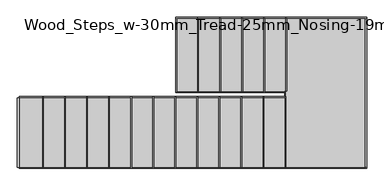
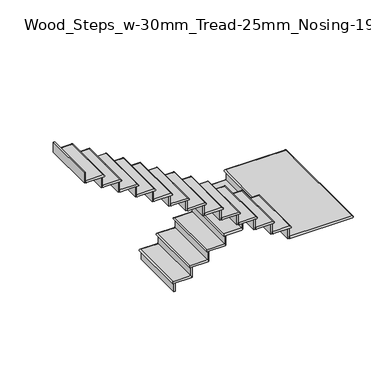
"""IFC4 building model written with IfcOpenShell, lengths in millimetres: stair flight geometry, Wood_Steps_w-30mm_Tread-25mm_Nosing-19mm_Riser."""

from ifc_helpers import new_model, si_unit, frame, origin, place, context, project, spatial, circle_curve, ellipse_curve, faceted_brep, source, transform, mapped, element, save
from ifc_brep_helpers import plane_surface, cylinder_surface, advanced_brep


def wood_steps_w_30mm_tread_25mm_nosing_19mm_riser_de9e5e1f(model_context):
    return source(origin(), model_context, "Body", "SolidModel", [
        advanced_brep(
        [(-8665.149573, -11058.3255223, 6797.52), (-8665.149573, -11058.3255223, 6827.52), (-8665.149573, -10219.6521308, 6827.52), (-8665.149573, -10219.6521308, 6797.52), (-8400.9545789, -11058.3255223, 6827.52), (-8400.9545789, -10219.6521308, 6827.52), (-8400.9545789, -10219.6521308, 6797.52), (-8400.9545789, -11058.3255223, 6797.52)],
        [
            (0, 1, ellipse_curve(frame((-8665.149573, -11058.3255223, 6812.52), z_axis=(-0.7071067811865475, 0.7071067811865475, 0.0), x_axis=(-0.7071067811865474, -0.7071067811865476, 0.0)), 21.2132034, 15.0)),
            (1, 2),
            (2, 3, ellipse_curve(frame((-8665.149573, -10219.6521308, 6812.52), z_axis=(-0.7071067811865475, -0.7071067811865475, 0.0), x_axis=(0.7071067811865474, -0.7071067811865476, 0.0)), 21.2132034, 15.0)),
            (3, 0),
            (4, 5),
            (5, 2),
            (1, 4),
            (6, 7),
            (7, 0),
            (3, 6),
            (4, 7, circle_curve(frame((-8400.9545789, -11058.3255223, 6812.52), z_axis=(1.0, 0.0, 0.0), x_axis=(0.0, 1.0, 0.0)), 15.0)),
            (6, 5, circle_curve(frame((-8400.9545789, -10219.6521308, 6812.52), z_axis=(1.0, 0.0, 0.0), x_axis=(0.0, -1.0, 0.0)), 15.0)),
        ],
        [
            cylinder_surface(frame((-8665.149573, -11058.3255223, 6812.52), z_axis=(0.0, -1.0, 0.0), x_axis=(1.0, 0.0, 0.0)), 15.0),
            plane_surface(frame((-6495.4132565, -10219.6521308, 6827.52), z_axis=(0.0, 0.0, 1.0), x_axis=(-1.0, 0.0, 0.0))),
            plane_surface(frame((-6495.4132565, -10219.6521308, 6797.52), z_axis=(0.0, 0.0, -1.0), x_axis=(1.0, 0.0, 0.0))),
            plane_surface(frame((-8400.9545789, -11058.3255223, 6827.52), z_axis=(1.0, 0.0, 0.0), x_axis=(0.0, 0.0, -1.0))),
            cylinder_surface(frame((-8400.9545789, -11058.3255223, 6812.52), z_axis=(1.0, 0.0, 0.0), x_axis=(0.0, 1.0, 0.0)), 15.0),
            cylinder_surface(frame((-8665.149573, -10219.6521308, 6812.52), z_axis=(-1.0, 0.0, 0.0), x_axis=(0.0, -1.0, 0.0)), 15.0),
        ],
        [
            (0, [[1, 2, 3, 4]]),
            (1, [[5, 6, -2, 7]]),
            (2, [[8, 9, -4, 10]]),
            (3, [[-5, 11, -8, 12]]),
            (4, [[-11, -7, -1, -9]]),
            (5, [[-3, -6, -12, -10]]),
        ],
    ),
        faceted_brep([(-8655.149573, -11058.3255223, 6797.52), (-8655.149573, -11058.3255223, 6664.96), (-8636.149573, -11058.3255223, 6664.96), (-8636.149573, -11058.3255223, 6797.52), (-8655.149573, -10219.6521308, 6797.52), (-8636.149573, -10219.6521308, 6797.52), (-8636.149573, -10219.6521308, 6664.96), (-8655.149573, -10219.6521308, 6664.96)], [[[0, 1, 2, 3]], [[4, 5, 6, 7]], [[1, 0, 4, 7]], [[2, 1, 7, 6]], [[3, 2, 6, 5]], [[0, 3, 5, 4]]]),
        faceted_brep([(-8400.9545789, -11058.3255223, 6960.08), (-8400.9545789, -11058.3255223, 6797.52), (-8381.9545789, -11058.3255223, 6797.52), (-8381.9545789, -11058.3255223, 6960.08), (-8400.9545789, -10219.6521308, 6960.08), (-8381.9545789, -10219.6521308, 6960.08), (-8381.9545789, -10219.6521308, 6797.52), (-8400.9545789, -10219.6521308, 6797.52)], [[[0, 1, 2, 3]], [[4, 5, 6, 7]], [[1, 0, 4, 7]], [[2, 1, 7, 6]], [[3, 2, 6, 5]], [[0, 3, 5, 4]]]),
        advanced_brep(
        [(-8146.7595849, -11058.3255223, 6990.08), (-8146.7595849, -10219.6521308, 6990.08), (-8410.9545789, -10219.6521308, 6990.08), (-8410.9545789, -11058.3255223, 6990.08), (-8146.7595849, -10219.6521308, 6960.08), (-8146.7595849, -11058.3255223, 6960.08), (-8410.9545789, -11058.3255223, 6960.08), (-8410.9545789, -10219.6521308, 6960.08)],
        [
            (0, 1),
            (1, 2),
            (2, 3),
            (3, 0),
            (4, 5),
            (5, 6),
            (6, 7),
            (7, 4),
            (0, 5, circle_curve(frame((-8146.7595849, -11058.3255223, 6975.08), z_axis=(1.0, 0.0, 0.0), x_axis=(0.0, 1.0, 0.0)), 15.0)),
            (4, 1, circle_curve(frame((-8146.7595849, -10219.6521308, 6975.08), z_axis=(1.0, 0.0, 0.0), x_axis=(0.0, -1.0, 0.0)), 15.0)),
            (6, 3, ellipse_curve(frame((-8410.9545789, -11058.3255223, 6975.08), z_axis=(-0.7071067811865475, 0.7071067811865475, 0.0), x_axis=(-0.7071067811865474, -0.7071067811865476, 0.0)), 21.2132034, 15.0)),
            (2, 7, ellipse_curve(frame((-8410.9545789, -10219.6521308, 6975.08), z_axis=(-0.7071067811865475, -0.7071067811865475, 0.0), x_axis=(0.7071067811865474, -0.7071067811865476, 0.0)), 21.2132034, 15.0)),
        ],
        [
            plane_surface(frame((-6495.4132565, -10219.6521308, 6990.08), z_axis=(0.0, 0.0, 1.0), x_axis=(-1.0, 0.0, 0.0))),
            plane_surface(frame((-6495.4132565, -10219.6521308, 6960.08), z_axis=(0.0, 0.0, -1.0), x_axis=(1.0, 0.0, 0.0))),
            plane_surface(frame((-8146.7595849, -11058.3255223, 6990.08), z_axis=(1.0, 0.0, 0.0), x_axis=(0.0, 0.0, -1.0))),
            cylinder_surface(frame((-8410.9545789, -11058.3255223, 6975.08), z_axis=(0.0, -1.0, 0.0), x_axis=(1.0, 0.0, 0.0)), 15.0),
            cylinder_surface(frame((-8146.7595849, -11058.3255223, 6975.08), z_axis=(1.0, 0.0, 0.0), x_axis=(0.0, 1.0, 0.0)), 15.0),
            cylinder_surface(frame((-8410.9545789, -10219.6521308, 6975.08), z_axis=(-1.0, 0.0, 0.0), x_axis=(0.0, -1.0, 0.0)), 15.0),
        ],
        [
            (0, [[1, 2, 3, 4]]),
            (1, [[5, 6, 7, 8]]),
            (2, [[-1, 9, -5, 10]]),
            (3, [[11, -3, 12, -7]]),
            (4, [[-9, -4, -11, -6]]),
            (5, [[-12, -2, -10, -8]]),
        ],
    ),
        faceted_brep([(-8146.7595849, -11058.3255223, 7122.64), (-8146.7595849, -11058.3255223, 6960.08), (-8127.7595849, -11058.3255223, 6960.08), (-8127.7595849, -11058.3255223, 7122.64), (-8146.7595849, -10219.6521308, 7122.64), (-8127.7595849, -10219.6521308, 7122.64), (-8127.7595849, -10219.6521308, 6960.08), (-8146.7595849, -10219.6521308, 6960.08)], [[[0, 1, 2, 3]], [[4, 5, 6, 7]], [[1, 0, 4, 7]], [[2, 1, 7, 6]], [[3, 2, 6, 5]], [[0, 3, 5, 4]]]),
        advanced_brep(
        [(-7893.1206135, -11058.3255223, 7152.64), (-7893.1206135, -10219.6521308, 7152.64), (-8156.7595849, -10219.6521308, 7152.64), (-8156.7595849, -11058.3255223, 7152.64), (-7893.1206135, -10219.6521308, 7122.64), (-7893.1206135, -11058.3255223, 7122.64), (-8156.7595849, -11058.3255223, 7122.64), (-8156.7595849, -10219.6521308, 7122.64)],
        [
            (0, 1),
            (1, 2),
            (2, 3),
            (3, 0),
            (4, 5),
            (5, 6),
            (6, 7),
            (7, 4),
            (0, 5, circle_curve(frame((-7893.1206135, -11058.3255223, 7137.64), z_axis=(1.0, 0.0, 0.0), x_axis=(0.0, 1.0, 0.0)), 15.0)),
            (4, 1, circle_curve(frame((-7893.1206135, -10219.6521308, 7137.64), z_axis=(1.0, 0.0, 0.0), x_axis=(0.0, -1.0, 0.0)), 15.0)),
            (6, 3, ellipse_curve(frame((-8156.7595849, -11058.3255223, 7137.64), z_axis=(-0.7071067811865475, 0.7071067811865475, 0.0), x_axis=(-0.7071067811865474, -0.7071067811865476, 0.0)), 21.2132034, 15.0)),
            (2, 7, ellipse_curve(frame((-8156.7595849, -10219.6521308, 7137.64), z_axis=(-0.7071067811865475, -0.7071067811865475, 0.0), x_axis=(0.7071067811865474, -0.7071067811865476, 0.0)), 21.2132034, 15.0)),
        ],
        [
            plane_surface(frame((-6495.4132565, -10219.6521308, 7152.64), z_axis=(0.0, 0.0, 1.0), x_axis=(-1.0, 0.0, 0.0))),
            plane_surface(frame((-6495.4132565, -10219.6521308, 7122.64), z_axis=(0.0, 0.0, -1.0), x_axis=(1.0, 0.0, 0.0))),
            plane_surface(frame((-7893.1206135, -11058.3255223, 7152.64), z_axis=(1.0, 0.0, 0.0), x_axis=(0.0, 0.0, -1.0))),
            cylinder_surface(frame((-8156.7595849, -11058.3255223, 7137.64), z_axis=(0.0, -1.0, 0.0), x_axis=(1.0, 0.0, 0.0)), 15.0),
            cylinder_surface(frame((-7893.1206135, -11058.3255223, 7137.64), z_axis=(1.0, 0.0, 0.0), x_axis=(0.0, 1.0, 0.0)), 15.0),
            cylinder_surface(frame((-8156.7595849, -10219.6521308, 7137.64), z_axis=(-1.0, 0.0, 0.0), x_axis=(0.0, -1.0, 0.0)), 15.0),
        ],
        [
            (0, [[1, 2, 3, 4]]),
            (1, [[5, 6, 7, 8]]),
            (2, [[-1, 9, -5, 10]]),
            (3, [[11, -3, 12, -7]]),
            (4, [[-9, -4, -11, -6]]),
            (5, [[-12, -2, -10, -8]]),
        ],
    ),
        faceted_brep([(-7893.1206135, -11058.3255223, 7285.2), (-7893.1206135, -11058.3255223, 7122.64), (-7874.1206135, -11058.3255223, 7122.64), (-7874.1206135, -11058.3255223, 7285.2), (-7893.1206135, -10219.6521308, 7285.2), (-7874.1206135, -10219.6521308, 7285.2), (-7874.1206135, -10219.6521308, 7122.64), (-7893.1206135, -10219.6521308, 7122.64)], [[[0, 1, 2, 3]], [[4, 5, 6, 7]], [[1, 0, 4, 7]], [[2, 1, 7, 6]], [[3, 2, 6, 5]], [[0, 3, 5, 4]]]),
        advanced_brep(
        [(-7638.9256194, -11058.3255223, 7315.2), (-7638.9256194, -10219.6521308, 7315.2), (-7903.1206135, -10219.6521308, 7315.2), (-7903.1206135, -11058.3255223, 7315.2), (-7638.9256194, -10219.6521308, 7285.2), (-7638.9256194, -11058.3255223, 7285.2), (-7903.1206135, -11058.3255223, 7285.2), (-7903.1206135, -10219.6521308, 7285.2)],
        [
            (0, 1),
            (1, 2),
            (2, 3),
            (3, 0),
            (4, 5),
            (5, 6),
            (6, 7),
            (7, 4),
            (0, 5, circle_curve(frame((-7638.9256194, -11058.3255223, 7300.2), z_axis=(1.0, 0.0, 0.0), x_axis=(0.0, 1.0, 0.0)), 15.0)),
            (4, 1, circle_curve(frame((-7638.9256194, -10219.6521308, 7300.2), z_axis=(1.0, 0.0, 0.0), x_axis=(0.0, -1.0, 0.0)), 15.0)),
            (6, 3, ellipse_curve(frame((-7903.1206135, -11058.3255223, 7300.2), z_axis=(-0.7071067811865475, 0.7071067811865475, 0.0), x_axis=(-0.7071067811865474, -0.7071067811865476, 0.0)), 21.2132034, 15.0)),
            (2, 7, ellipse_curve(frame((-7903.1206135, -10219.6521308, 7300.2), z_axis=(-0.7071067811865475, -0.7071067811865475, 0.0), x_axis=(0.7071067811865474, -0.7071067811865476, 0.0)), 21.2132034, 15.0)),
        ],
        [
            plane_surface(frame((-6495.4132565, -10219.6521308, 7315.2), z_axis=(0.0, 0.0, 1.0), x_axis=(-1.0, 0.0, 0.0))),
            plane_surface(frame((-6495.4132565, -10219.6521308, 7285.2), z_axis=(0.0, 0.0, -1.0), x_axis=(1.0, 0.0, 0.0))),
            plane_surface(frame((-7638.9256194, -11058.3255223, 7315.2), z_axis=(1.0, 0.0, 0.0), x_axis=(0.0, 0.0, -1.0))),
            cylinder_surface(frame((-7903.1206135, -11058.3255223, 7300.2), z_axis=(0.0, -1.0, 0.0), x_axis=(1.0, 0.0, 0.0)), 15.0),
            cylinder_surface(frame((-7638.9256194, -11058.3255223, 7300.2), z_axis=(1.0, 0.0, 0.0), x_axis=(0.0, 1.0, 0.0)), 15.0),
            cylinder_surface(frame((-7903.1206135, -10219.6521308, 7300.2), z_axis=(-1.0, 0.0, 0.0), x_axis=(0.0, -1.0, 0.0)), 15.0),
        ],
        [
            (0, [[1, 2, 3, 4]]),
            (1, [[5, 6, 7, 8]]),
            (2, [[-1, 9, -5, 10]]),
            (3, [[11, -3, 12, -7]]),
            (4, [[-9, -4, -11, -6]]),
            (5, [[-12, -2, -10, -8]]),
        ],
    ),
        faceted_brep([(-7384.7306254, -11058.3255223, 7610.32), (-7384.7306254, -11058.3255223, 7447.76), (-7365.7306254, -11058.3255223, 7447.76), (-7365.7306254, -11058.3255223, 7610.32), (-7384.7306254, -10219.6521308, 7610.32), (-7365.7306254, -10219.6521308, 7610.32), (-7365.7306254, -10219.6521308, 7447.76), (-7384.7306254, -10219.6521308, 7447.76)], [[[0, 1, 2, 3]], [[4, 5, 6, 7]], [[1, 0, 4, 7]], [[2, 1, 7, 6]], [[3, 2, 6, 5]], [[0, 3, 5, 4]]]),
        faceted_brep([(-7434.7306254, -11134.5255223, 7772.88), (-7434.7306254, -11134.5255223, 7610.32), (-7453.7306254, -11134.5255223, 7610.32), (-7453.7306254, -11134.5255223, 7772.88), (-7434.7306254, -11934.0860066, 7772.88), (-7453.7306254, -11934.0860066, 7772.88), (-7453.7306254, -11934.0860066, 7610.32), (-7434.7306254, -11934.0860066, 7610.32)], [[[0, 1, 2, 3]], [[4, 5, 6, 7]], [[1, 0, 4, 7]], [[2, 1, 7, 6]], [[3, 2, 6, 5]], [[0, 3, 5, 4]]]),
        advanced_brep(
        [(-7688.9256194, -11134.5255223, 7802.88), (-7688.9256194, -11934.0860066, 7802.88), (-7424.7306254, -11934.0860066, 7802.88), (-7424.7306254, -11134.5255223, 7802.88), (-7688.9256194, -11934.0860066, 7772.88), (-7688.9256194, -11134.5255223, 7772.88), (-7424.7306254, -11134.5255223, 7772.88), (-7424.7306254, -11934.0860066, 7772.88)],
        [
            (0, 1),
            (1, 2),
            (2, 3),
            (3, 0),
            (4, 5),
            (5, 6),
            (6, 7),
            (7, 4),
            (0, 5, circle_curve(frame((-7688.9256194, -11134.5255223, 7787.88), z_axis=(-1.0, 0.0, 0.0), x_axis=(0.0, -1.0, 0.0)), 15.0)),
            (4, 1, circle_curve(frame((-7688.9256194, -11934.0860066, 7787.88), z_axis=(-1.0, 0.0, 0.0), x_axis=(0.0, 1.0, 0.0)), 15.0)),
            (6, 3, ellipse_curve(frame((-7424.7306254, -11134.5255223, 7787.88), z_axis=(0.7071067811865475, -0.7071067811865475, 0.0), x_axis=(0.7071067811865474, 0.7071067811865476, 0.0)), 21.2132034, 15.0)),
            (2, 7, ellipse_curve(frame((-7424.7306254, -11934.0860066, 7787.88), z_axis=(0.7071067811865475, 0.7071067811865475, 0.0), x_axis=(-0.7071067811865474, 0.7071067811865476, 0.0)), 21.2132034, 15.0)),
        ],
        [
            plane_surface(frame((-10457.8773536, -11934.0860066, 7802.88), z_axis=(0.0, 0.0, 1.0), x_axis=(1.0, 0.0, 0.0))),
            plane_surface(frame((-10457.8773536, -11934.0860066, 7772.88), z_axis=(0.0, 0.0, -1.0), x_axis=(-1.0, 0.0, 0.0))),
            plane_surface(frame((-7688.9256194, -11134.5255223, 7802.88), z_axis=(-1.0, 0.0, 0.0), x_axis=(0.0, 0.0, -1.0))),
            cylinder_surface(frame((-7424.7306254, -11134.5255223, 7787.88), z_axis=(0.0, 1.0, 0.0), x_axis=(-1.0, 0.0, 0.0)), 15.0),
            cylinder_surface(frame((-7688.9256194, -11134.5255223, 7787.88), z_axis=(-1.0, 0.0, 0.0), x_axis=(0.0, -1.0, 0.0)), 15.0),
            cylinder_surface(frame((-7424.7306254, -11934.0860066, 7787.88), z_axis=(1.0, 0.0, 0.0), x_axis=(0.0, 1.0, 0.0)), 15.0),
        ],
        [
            (0, [[1, 2, 3, 4]]),
            (1, [[5, 6, 7, 8]]),
            (2, [[-1, 9, -5, 10]]),
            (3, [[11, -3, 12, -7]]),
            (4, [[-9, -4, -11, -6]]),
            (5, [[-12, -2, -10, -8]]),
        ],
    ),
        faceted_brep([(-8196.7595849, -11134.5255223, 8260.56), (-8196.7595849, -11134.5255223, 8098.0), (-8215.7595849, -11134.5255223, 8098.0), (-8215.7595849, -11134.5255223, 8260.56), (-8196.7595849, -11934.0860066, 8260.56), (-8215.7595849, -11934.0860066, 8260.56), (-8215.7595849, -11934.0860066, 8098.0), (-8196.7595849, -11934.0860066, 8098.0)], [[[0, 1, 2, 3]], [[4, 5, 6, 7]], [[1, 0, 4, 7]], [[2, 1, 7, 6]], [[3, 2, 6, 5]], [[0, 3, 5, 4]]]),
        advanced_brep(
        [(-8450.9545789, -11134.5255223, 8290.56), (-8450.9545789, -11934.0860066, 8290.56), (-8186.7595849, -11934.0860066, 8290.56), (-8186.7595849, -11134.5255223, 8290.56), (-8450.9545789, -11934.0860066, 8260.56), (-8450.9545789, -11134.5255223, 8260.56), (-8186.7595849, -11134.5255223, 8260.56), (-8186.7595849, -11934.0860066, 8260.56)],
        [
            (0, 1),
            (1, 2),
            (2, 3),
            (3, 0),
            (4, 5),
            (5, 6),
            (6, 7),
            (7, 4),
            (0, 5, circle_curve(frame((-8450.9545789, -11134.5255223, 8275.56), z_axis=(-1.0, 0.0, 0.0), x_axis=(0.0, -1.0, 0.0)), 15.0)),
            (4, 1, circle_curve(frame((-8450.9545789, -11934.0860066, 8275.56), z_axis=(-1.0, 0.0, 0.0), x_axis=(0.0, 1.0, 0.0)), 15.0)),
            (6, 3, ellipse_curve(frame((-8186.7595849, -11134.5255223, 8275.56), z_axis=(0.7071067811865475, -0.7071067811865475, 0.0), x_axis=(0.7071067811865474, 0.7071067811865476, 0.0)), 21.2132034, 15.0)),
            (2, 7, ellipse_curve(frame((-8186.7595849, -11934.0860066, 8275.56), z_axis=(0.7071067811865475, 0.7071067811865475, 0.0), x_axis=(-0.7071067811865474, 0.7071067811865476, 0.0)), 21.2132034, 15.0)),
        ],
        [
            plane_surface(frame((-10457.8773536, -11934.0860066, 8290.56), z_axis=(0.0, 0.0, 1.0), x_axis=(1.0, 0.0, 0.0))),
            plane_surface(frame((-10457.8773536, -11934.0860066, 8260.56), z_axis=(0.0, 0.0, -1.0), x_axis=(-1.0, 0.0, 0.0))),
            plane_surface(frame((-8450.9545789, -11134.5255223, 8290.56), z_axis=(-1.0, 0.0, 0.0), x_axis=(0.0, 0.0, -1.0))),
            cylinder_surface(frame((-8186.7595849, -11134.5255223, 8275.56), z_axis=(0.0, 1.0, 0.0), x_axis=(-1.0, 0.0, 0.0)), 15.0),
            cylinder_surface(frame((-8450.9545789, -11134.5255223, 8275.56), z_axis=(-1.0, 0.0, 0.0), x_axis=(0.0, -1.0, 0.0)), 15.0),
            cylinder_surface(frame((-8186.7595849, -11934.0860066, 8275.56), z_axis=(1.0, 0.0, 0.0), x_axis=(0.0, 1.0, 0.0)), 15.0),
        ],
        [
            (0, [[1, 2, 3, 4]]),
            (1, [[5, 6, 7, 8]]),
            (2, [[-1, 9, -5, 10]]),
            (3, [[11, -3, 12, -7]]),
            (4, [[-9, -4, -11, -6]]),
            (5, [[-12, -2, -10, -8]]),
        ],
    ),
        faceted_brep([(-8958.7885444, -11134.5255223, 8748.24), (-8958.7885444, -11134.5255223, 8585.68), (-8977.7885444, -11134.5255223, 8585.68), (-8977.7885444, -11134.5255223, 8748.24), (-8958.7885444, -11934.0860066, 8748.24), (-8977.7885444, -11934.0860066, 8748.24), (-8977.7885444, -11934.0860066, 8585.68), (-8958.7885444, -11934.0860066, 8585.68)], [[[0, 1, 2, 3]], [[4, 5, 6, 7]], [[1, 0, 4, 7]], [[2, 1, 7, 6]], [[3, 2, 6, 5]], [[0, 3, 5, 4]]]),
        advanced_brep(
        [(-9212.9835384, -11134.5255223, 8778.24), (-9212.9835384, -11934.0860066, 8778.24), (-8948.7885444, -11934.0860066, 8778.24), (-8948.7885444, -11134.5255223, 8778.24), (-9212.9835384, -11934.0860066, 8748.24), (-9212.9835384, -11134.5255223, 8748.24), (-8948.7885444, -11134.5255223, 8748.24), (-8948.7885444, -11934.0860066, 8748.24)],
        [
            (0, 1),
            (1, 2),
            (2, 3),
            (3, 0),
            (4, 5),
            (5, 6),
            (6, 7),
            (7, 4),
            (0, 5, circle_curve(frame((-9212.9835384, -11134.5255223, 8763.24), z_axis=(-1.0, 0.0, 0.0), x_axis=(0.0, -1.0, 0.0)), 15.0)),
            (4, 1, circle_curve(frame((-9212.9835384, -11934.0860066, 8763.24), z_axis=(-1.0, 0.0, 0.0), x_axis=(0.0, 1.0, 0.0)), 15.0)),
            (6, 3, ellipse_curve(frame((-8948.7885444, -11134.5255223, 8763.24), z_axis=(0.7071067811865475, -0.7071067811865475, 0.0), x_axis=(0.7071067811865474, 0.7071067811865476, 0.0)), 21.2132034, 15.0)),
            (2, 7, ellipse_curve(frame((-8948.7885444, -11934.0860066, 8763.24), z_axis=(0.7071067811865475, 0.7071067811865475, 0.0), x_axis=(-0.7071067811865474, 0.7071067811865476, 0.0)), 21.2132034, 15.0)),
        ],
        [
            plane_surface(frame((-10457.8773536, -11934.0860066, 8778.24), z_axis=(0.0, 0.0, 1.0), x_axis=(1.0, 0.0, 0.0))),
            plane_surface(frame((-10457.8773536, -11934.0860066, 8748.24), z_axis=(0.0, 0.0, -1.0), x_axis=(-1.0, 0.0, 0.0))),
            plane_surface(frame((-9212.9835384, -11134.5255223, 8778.24), z_axis=(-1.0, 0.0, 0.0), x_axis=(0.0, 0.0, -1.0))),
            cylinder_surface(frame((-8948.7885444, -11134.5255223, 8763.24), z_axis=(0.0, 1.0, 0.0), x_axis=(-1.0, 0.0, 0.0)), 15.0),
            cylinder_surface(frame((-9212.9835384, -11134.5255223, 8763.24), z_axis=(-1.0, 0.0, 0.0), x_axis=(0.0, -1.0, 0.0)), 15.0),
            cylinder_surface(frame((-8948.7885444, -11934.0860066, 8763.24), z_axis=(1.0, 0.0, 0.0), x_axis=(0.0, 1.0, 0.0)), 15.0),
        ],
        [
            (0, [[1, 2, 3, 4]]),
            (1, [[5, 6, 7, 8]]),
            (2, [[-1, 9, -5, 10]]),
            (3, [[11, -3, 12, -7]]),
            (4, [[-9, -4, -11, -6]]),
            (5, [[-12, -2, -10, -8]]),
        ],
    ),
        faceted_brep([(-9212.9835384, -11134.5255223, 8910.8), (-9212.9835384, -11134.5255223, 8748.24), (-9231.9835384, -11134.5255223, 8748.24), (-9231.9835384, -11134.5255223, 8910.8), (-9212.9835384, -11934.0860066, 8910.8), (-9231.9835384, -11934.0860066, 8910.8), (-9231.9835384, -11934.0860066, 8748.24), (-9212.9835384, -11934.0860066, 8748.24)], [[[0, 1, 2, 3]], [[4, 5, 6, 7]], [[1, 0, 4, 7]], [[2, 1, 7, 6]], [[3, 2, 6, 5]], [[0, 3, 5, 4]]]),
        advanced_brep(
        [(-9466.6534, -11134.5255223, 8940.8), (-9466.6534, -11934.0860066, 8940.8), (-9202.9835384, -11934.0860066, 8940.8), (-9202.9835384, -11134.5255223, 8940.8), (-9466.6534, -11934.0860066, 8910.8), (-9466.6534, -11134.5255223, 8910.8), (-9202.9835384, -11134.5255223, 8910.8), (-9202.9835384, -11934.0860066, 8910.8)],
        [
            (0, 1),
            (1, 2),
            (2, 3),
            (3, 0),
            (4, 5),
            (5, 6),
            (6, 7),
            (7, 4),
            (0, 5, circle_curve(frame((-9466.6534, -11134.5255223, 8925.8), z_axis=(-1.0, 0.0, 0.0), x_axis=(0.0, -1.0, 0.0)), 15.0)),
            (4, 1, circle_curve(frame((-9466.6534, -11934.0860066, 8925.8), z_axis=(-1.0, 0.0, 0.0), x_axis=(0.0, 1.0, 0.0)), 15.0)),
            (6, 3, ellipse_curve(frame((-9202.9835384, -11134.5255223, 8925.8), z_axis=(0.7071067811865475, -0.7071067811865475, 0.0), x_axis=(0.7071067811865474, 0.7071067811865476, 0.0)), 21.2132034, 15.0)),
            (2, 7, ellipse_curve(frame((-9202.9835384, -11934.0860066, 8925.8), z_axis=(0.7071067811865475, 0.7071067811865475, 0.0), x_axis=(-0.7071067811865474, 0.7071067811865476, 0.0)), 21.2132034, 15.0)),
        ],
        [
            plane_surface(frame((-10457.8773536, -11934.0860066, 8940.8), z_axis=(0.0, 0.0, 1.0), x_axis=(1.0, 0.0, 0.0))),
            plane_surface(frame((-10457.8773536, -11934.0860066, 8910.8), z_axis=(0.0, 0.0, -1.0), x_axis=(-1.0, 0.0, 0.0))),
            plane_surface(frame((-9466.6534, -11134.5255223, 8940.8), z_axis=(-1.0, 0.0, 0.0), x_axis=(0.0, 0.0, -1.0))),
            cylinder_surface(frame((-9202.9835384, -11134.5255223, 8925.8), z_axis=(0.0, 1.0, 0.0), x_axis=(-1.0, 0.0, 0.0)), 15.0),
            cylinder_surface(frame((-9466.6534, -11134.5255223, 8925.8), z_axis=(-1.0, 0.0, 0.0), x_axis=(0.0, -1.0, 0.0)), 15.0),
            cylinder_surface(frame((-9202.9835384, -11934.0860066, 8925.8), z_axis=(1.0, 0.0, 0.0), x_axis=(0.0, 1.0, 0.0)), 15.0),
        ],
        [
            (0, [[1, 2, 3, 4]]),
            (1, [[5, 6, 7, 8]]),
            (2, [[-1, 9, -5, 10]]),
            (3, [[11, -3, 12, -7]]),
            (4, [[-9, -4, -11, -6]]),
            (5, [[-12, -2, -10, -8]]),
        ],
    ),
        faceted_brep([(-9720.8175039, -11134.5255223, 9235.92), (-9720.8175039, -11134.5255223, 9073.36), (-9739.8175039, -11134.5255223, 9073.36), (-9739.8175039, -11134.5255223, 9235.92), (-9720.8175039, -11934.0860066, 9235.92), (-9739.8175039, -11934.0860066, 9235.92), (-9739.8175039, -11934.0860066, 9073.36), (-9720.8175039, -11934.0860066, 9073.36)], [[[0, 1, 2, 3]], [[4, 5, 6, 7]], [[1, 0, 4, 7]], [[2, 1, 7, 6]], [[3, 2, 6, 5]], [[0, 3, 5, 4]]]),
        advanced_brep(
        [(-9975.012498, -11134.5255223, 9265.92), (-9975.012498, -11934.0860066, 9265.92), (-9710.8175039, -11934.0860066, 9265.92), (-9710.8175039, -11134.5255223, 9265.92), (-9975.012498, -11934.0860066, 9235.92), (-9975.012498, -11134.5255223, 9235.92), (-9710.8175039, -11134.5255223, 9235.92), (-9710.8175039, -11934.0860066, 9235.92)],
        [
            (0, 1),
            (1, 2),
            (2, 3),
            (3, 0),
            (4, 5),
            (5, 6),
            (6, 7),
            (7, 4),
            (0, 5, circle_curve(frame((-9975.012498, -11134.5255223, 9250.92), z_axis=(-1.0, 0.0, 0.0), x_axis=(0.0, -1.0, 0.0)), 15.0)),
            (4, 1, circle_curve(frame((-9975.012498, -11934.0860066, 9250.92), z_axis=(-1.0, 0.0, 0.0), x_axis=(0.0, 1.0, 0.0)), 15.0)),
            (6, 3, ellipse_curve(frame((-9710.8175039, -11134.5255223, 9250.92), z_axis=(0.7071067811865475, -0.7071067811865475, 0.0), x_axis=(0.7071067811865474, 0.7071067811865476, 0.0)), 21.2132034, 15.0)),
            (2, 7, ellipse_curve(frame((-9710.8175039, -11934.0860066, 9250.92), z_axis=(0.7071067811865475, 0.7071067811865475, 0.0), x_axis=(-0.7071067811865474, 0.7071067811865476, 0.0)), 21.2132034, 15.0)),
        ],
        [
            plane_surface(frame((-10457.8773536, -11934.0860066, 9265.92), z_axis=(0.0, 0.0, 1.0), x_axis=(1.0, 0.0, 0.0))),
            plane_surface(frame((-10457.8773536, -11934.0860066, 9235.92), z_axis=(0.0, 0.0, -1.0), x_axis=(-1.0, 0.0, 0.0))),
            plane_surface(frame((-9975.012498, -11134.5255223, 9265.92), z_axis=(-1.0, 0.0, 0.0), x_axis=(0.0, 0.0, -1.0))),
            cylinder_surface(frame((-9710.8175039, -11134.5255223, 9250.92), z_axis=(0.0, 1.0, 0.0), x_axis=(-1.0, 0.0, 0.0)), 15.0),
            cylinder_surface(frame((-9975.012498, -11134.5255223, 9250.92), z_axis=(-1.0, 0.0, 0.0), x_axis=(0.0, -1.0, 0.0)), 15.0),
            cylinder_surface(frame((-9710.8175039, -11934.0860066, 9250.92), z_axis=(1.0, 0.0, 0.0), x_axis=(0.0, 1.0, 0.0)), 15.0),
        ],
        [
            (0, [[1, 2, 3, 4]]),
            (1, [[5, 6, 7, 8]]),
            (2, [[-1, 9, -5, 10]]),
            (3, [[11, -3, 12, -7]]),
            (4, [[-9, -4, -11, -6]]),
            (5, [[-12, -2, -10, -8]]),
        ],
    ),
        faceted_brep([(-9975.012498, -11134.5255223, 9398.48), (-9975.012498, -11134.5255223, 9235.92), (-9994.012498, -11134.5255223, 9235.92), (-9994.012498, -11134.5255223, 9398.48), (-9975.012498, -11934.0860066, 9398.48), (-9994.012498, -11934.0860066, 9398.48), (-9994.012498, -11934.0860066, 9235.92), (-9975.012498, -11934.0860066, 9235.92)], [[[0, 1, 2, 3]], [[4, 5, 6, 7]], [[1, 0, 4, 7]], [[2, 1, 7, 6]], [[3, 2, 6, 5]], [[0, 3, 5, 4]]]),
        advanced_brep(
        [(-10228.6823595, -11134.5255223, 9428.48), (-10228.6823595, -11934.0860066, 9428.48), (-9965.012498, -11934.0860066, 9428.48), (-9965.012498, -11134.5255223, 9428.48), (-10228.6823595, -11934.0860066, 9398.48), (-10228.6823595, -11134.5255223, 9398.48), (-9965.012498, -11134.5255223, 9398.48), (-9965.012498, -11934.0860066, 9398.48)],
        [
            (0, 1),
            (1, 2),
            (2, 3),
            (3, 0),
            (4, 5),
            (5, 6),
            (6, 7),
            (7, 4),
            (0, 5, circle_curve(frame((-10228.6823595, -11134.5255223, 9413.48), z_axis=(-1.0, 0.0, 0.0), x_axis=(0.0, -1.0, 0.0)), 15.0)),
            (4, 1, circle_curve(frame((-10228.6823595, -11934.0860066, 9413.48), z_axis=(-1.0, 0.0, 0.0), x_axis=(0.0, 1.0, 0.0)), 15.0)),
            (6, 3, ellipse_curve(frame((-9965.012498, -11134.5255223, 9413.48), z_axis=(0.7071067811865475, -0.7071067811865475, 0.0), x_axis=(0.7071067811865474, 0.7071067811865476, 0.0)), 21.2132034, 15.0)),
            (2, 7, ellipse_curve(frame((-9965.012498, -11934.0860066, 9413.48), z_axis=(0.7071067811865475, 0.7071067811865475, 0.0), x_axis=(-0.7071067811865474, 0.7071067811865476, 0.0)), 21.2132034, 15.0)),
        ],
        [
            plane_surface(frame((-10457.8773536, -11934.0860066, 9428.48), z_axis=(0.0, 0.0, 1.0), x_axis=(1.0, 0.0, 0.0))),
            plane_surface(frame((-10457.8773536, -11934.0860066, 9398.48), z_axis=(0.0, 0.0, -1.0), x_axis=(-1.0, 0.0, 0.0))),
            plane_surface(frame((-10228.6823595, -11134.5255223, 9428.48), z_axis=(-1.0, 0.0, 0.0), x_axis=(0.0, 0.0, -1.0))),
            cylinder_surface(frame((-9965.012498, -11134.5255223, 9413.48), z_axis=(0.0, 1.0, 0.0), x_axis=(-1.0, 0.0, 0.0)), 15.0),
            cylinder_surface(frame((-10228.6823595, -11134.5255223, 9413.48), z_axis=(-1.0, 0.0, 0.0), x_axis=(0.0, -1.0, 0.0)), 15.0),
            cylinder_surface(frame((-9965.012498, -11934.0860066, 9413.48), z_axis=(1.0, 0.0, 0.0), x_axis=(0.0, 1.0, 0.0)), 15.0),
        ],
        [
            (0, [[1, 2, 3, 4]]),
            (1, [[5, 6, 7, 8]]),
            (2, [[-1, 9, -5, 10]]),
            (3, [[11, -3, 12, -7]]),
            (4, [[-9, -4, -11, -6]]),
            (5, [[-12, -2, -10, -8]]),
        ],
    ),
        faceted_brep([(-10482.8773536, -11134.5255223, 9723.6), (-10482.8773536, -11134.5255223, 9561.04), (-10501.8773536, -11134.5255223, 9561.04), (-10501.8773536, -11134.5255223, 9723.6), (-10482.8773536, -11934.0860066, 9723.6), (-10501.8773536, -11934.0860066, 9723.6), (-10501.8773536, -11934.0860066, 9561.04), (-10482.8773536, -11934.0860066, 9561.04)], [[[0, 1, 2, 3]], [[4, 5, 6, 7]], [[1, 0, 4, 7]], [[2, 1, 7, 6]], [[3, 2, 6, 5]], [[0, 3, 5, 4]]]),
        faceted_brep([(-7638.9256194, -11058.3255223, 7447.76), (-7638.9256194, -11058.3255223, 7285.2), (-7619.9256194, -11058.3255223, 7285.2), (-7619.9256194, -11058.3255223, 7447.76), (-7638.9256194, -10219.6521308, 7447.76), (-7619.9256194, -10219.6521308, 7447.76), (-7619.9256194, -10219.6521308, 7285.2), (-7638.9256194, -10219.6521308, 7285.2)], [[[0, 1, 2, 3]], [[4, 5, 6, 7]], [[1, 0, 4, 7]], [[2, 1, 7, 6]], [[3, 2, 6, 5]], [[0, 3, 5, 4]]]),
        advanced_brep(
        [(-7384.7306254, -11058.3255223, 7477.76), (-7384.7306254, -10219.6521308, 7477.76), (-7648.9256194, -10219.6521308, 7477.76), (-7648.9256194, -11058.3255223, 7477.76), (-7384.7306254, -10219.6521308, 7447.76), (-7384.7306254, -11058.3255223, 7447.76), (-7648.9256194, -11058.3255223, 7447.76), (-7648.9256194, -10219.6521308, 7447.76)],
        [
            (0, 1),
            (1, 2),
            (2, 3),
            (3, 0),
            (4, 5),
            (5, 6),
            (6, 7),
            (7, 4),
            (0, 5, circle_curve(frame((-7384.7306254, -11058.3255223, 7462.76), z_axis=(1.0, 0.0, 0.0), x_axis=(0.0, 1.0, 0.0)), 15.0)),
            (4, 1, circle_curve(frame((-7384.7306254, -10219.6521308, 7462.76), z_axis=(1.0, 0.0, 0.0), x_axis=(0.0, -1.0, 0.0)), 15.0)),
            (6, 3, ellipse_curve(frame((-7648.9256194, -11058.3255223, 7462.76), z_axis=(-0.7071067811865475, 0.7071067811865475, 0.0), x_axis=(-0.7071067811865474, -0.7071067811865476, 0.0)), 21.2132034, 15.0)),
            (2, 7, ellipse_curve(frame((-7648.9256194, -10219.6521308, 7462.76), z_axis=(-0.7071067811865475, -0.7071067811865475, 0.0), x_axis=(0.7071067811865474, -0.7071067811865476, 0.0)), 21.2132034, 15.0)),
        ],
        [
            plane_surface(frame((-6241.2182625, -10219.6521308, 7477.76), z_axis=(0.0, 0.0, 1.0), x_axis=(-1.0, 0.0, 0.0))),
            plane_surface(frame((-6241.2182625, -10219.6521308, 7447.76), z_axis=(0.0, 0.0, -1.0), x_axis=(1.0, 0.0, 0.0))),
            plane_surface(frame((-7384.7306254, -11058.3255223, 7477.76), z_axis=(1.0, 0.0, 0.0), x_axis=(0.0, 0.0, -1.0))),
            cylinder_surface(frame((-7648.9256194, -11058.3255223, 7462.76), z_axis=(0.0, -1.0, 0.0), x_axis=(1.0, 0.0, 0.0)), 15.0),
            cylinder_surface(frame((-7384.7306254, -11058.3255223, 7462.76), z_axis=(1.0, 0.0, 0.0), x_axis=(0.0, 1.0, 0.0)), 15.0),
            cylinder_surface(frame((-7648.9256194, -10219.6521308, 7462.76), z_axis=(-1.0, 0.0, 0.0), x_axis=(0.0, -1.0, 0.0)), 15.0),
        ],
        [
            (0, [[1, 2, 3, 4]]),
            (1, [[5, 6, 7, 8]]),
            (2, [[-1, 9, -5, 10]]),
            (3, [[11, -3, 12, -7]]),
            (4, [[-9, -4, -11, -6]]),
            (5, [[-12, -2, -10, -8]]),
        ],
    ),
        faceted_brep([(-7688.9256194, -11134.5255223, 7935.44), (-7688.9256194, -11134.5255223, 7772.88), (-7707.9256194, -11134.5255223, 7772.88), (-7707.9256194, -11134.5255223, 7935.44), (-7688.9256194, -11934.0860066, 7935.44), (-7707.9256194, -11934.0860066, 7935.44), (-7707.9256194, -11934.0860066, 7772.88), (-7688.9256194, -11934.0860066, 7772.88)], [[[0, 1, 2, 3]], [[4, 5, 6, 7]], [[1, 0, 4, 7]], [[2, 1, 7, 6]], [[3, 2, 6, 5]], [[0, 3, 5, 4]]]),
        advanced_brep(
        [(-7943.1206135, -11134.5255223, 7965.44), (-7943.1206135, -11934.0860066, 7965.44), (-7678.9256194, -11934.0860066, 7965.44), (-7678.9256194, -11134.5255223, 7965.44), (-7943.1206135, -11934.0860066, 7935.44), (-7943.1206135, -11134.5255223, 7935.44), (-7678.9256194, -11134.5255223, 7935.44), (-7678.9256194, -11934.0860066, 7935.44)],
        [
            (0, 1),
            (1, 2),
            (2, 3),
            (3, 0),
            (4, 5),
            (5, 6),
            (6, 7),
            (7, 4),
            (0, 5, circle_curve(frame((-7943.1206135, -11134.5255223, 7950.44), z_axis=(-1.0, 0.0, 0.0), x_axis=(0.0, -1.0, 0.0)), 15.0)),
            (4, 1, circle_curve(frame((-7943.1206135, -11934.0860066, 7950.44), z_axis=(-1.0, 0.0, 0.0), x_axis=(0.0, 1.0, 0.0)), 15.0)),
            (6, 3, ellipse_curve(frame((-7678.9256194, -11134.5255223, 7950.44), z_axis=(0.7071067811865475, -0.7071067811865475, 0.0), x_axis=(0.7071067811865474, 0.7071067811865476, 0.0)), 21.2132034, 15.0)),
            (2, 7, ellipse_curve(frame((-7678.9256194, -11934.0860066, 7950.44), z_axis=(0.7071067811865475, 0.7071067811865475, 0.0), x_axis=(-0.7071067811865474, 0.7071067811865476, 0.0)), 21.2132034, 15.0)),
        ],
        [
            plane_surface(frame((-10712.0723476, -11934.0860066, 7965.44), z_axis=(0.0, 0.0, 1.0), x_axis=(1.0, 0.0, 0.0))),
            plane_surface(frame((-10712.0723476, -11934.0860066, 7935.44), z_axis=(0.0, 0.0, -1.0), x_axis=(-1.0, 0.0, 0.0))),
            plane_surface(frame((-7943.1206135, -11134.5255223, 7965.44), z_axis=(-1.0, 0.0, 0.0), x_axis=(0.0, 0.0, -1.0))),
            cylinder_surface(frame((-7678.9256194, -11134.5255223, 7950.44), z_axis=(0.0, 1.0, 0.0), x_axis=(-1.0, 0.0, 0.0)), 15.0),
            cylinder_surface(frame((-7943.1206135, -11134.5255223, 7950.44), z_axis=(-1.0, 0.0, 0.0), x_axis=(0.0, -1.0, 0.0)), 15.0),
            cylinder_surface(frame((-7678.9256194, -11934.0860066, 7950.44), z_axis=(1.0, 0.0, 0.0), x_axis=(0.0, 1.0, 0.0)), 15.0),
        ],
        [
            (0, [[1, 2, 3, 4]]),
            (1, [[5, 6, 7, 8]]),
            (2, [[-1, 9, -5, 10]]),
            (3, [[11, -3, 12, -7]]),
            (4, [[-9, -4, -11, -6]]),
            (5, [[-12, -2, -10, -8]]),
        ],
    ),
        faceted_brep([(-7943.1206135, -11134.5255223, 8098.0), (-7943.1206135, -11134.5255223, 7935.44), (-7962.1206135, -11134.5255223, 7935.44), (-7962.1206135, -11134.5255223, 8098.0), (-7943.1206135, -11934.0860066, 8098.0), (-7962.1206135, -11934.0860066, 8098.0), (-7962.1206135, -11934.0860066, 7935.44), (-7943.1206135, -11934.0860066, 7935.44)], [[[0, 1, 2, 3]], [[4, 5, 6, 7]], [[1, 0, 4, 7]], [[2, 1, 7, 6]], [[3, 2, 6, 5]], [[0, 3, 5, 4]]]),
        advanced_brep(
        [(-8196.7595849, -11134.5255223, 8128.0), (-8196.7595849, -11934.0860066, 8128.0), (-7933.1206135, -11934.0860066, 8128.0), (-7933.1206135, -11134.5255223, 8128.0), (-8196.7595849, -11934.0860066, 8098.0), (-8196.7595849, -11134.5255223, 8098.0), (-7933.1206135, -11134.5255223, 8098.0), (-7933.1206135, -11934.0860066, 8098.0)],
        [
            (0, 1),
            (1, 2),
            (2, 3),
            (3, 0),
            (4, 5),
            (5, 6),
            (6, 7),
            (7, 4),
            (0, 5, circle_curve(frame((-8196.7595849, -11134.5255223, 8113.0), z_axis=(-1.0, 0.0, 0.0), x_axis=(0.0, -1.0, 0.0)), 15.0)),
            (4, 1, circle_curve(frame((-8196.7595849, -11934.0860066, 8113.0), z_axis=(-1.0, 0.0, 0.0), x_axis=(0.0, 1.0, 0.0)), 15.0)),
            (6, 3, ellipse_curve(frame((-7933.1206135, -11134.5255223, 8113.0), z_axis=(0.7071067811865475, -0.7071067811865475, 0.0), x_axis=(0.7071067811865474, 0.7071067811865476, 0.0)), 21.2132034, 15.0)),
            (2, 7, ellipse_curve(frame((-7933.1206135, -11934.0860066, 8113.0), z_axis=(0.7071067811865475, 0.7071067811865475, 0.0), x_axis=(-0.7071067811865474, 0.7071067811865476, 0.0)), 21.2132034, 15.0)),
        ],
        [
            plane_surface(frame((-10457.8773536, -11934.0860066, 8128.0), z_axis=(0.0, 0.0, 1.0), x_axis=(1.0, 0.0, 0.0))),
            plane_surface(frame((-10457.8773536, -11934.0860066, 8098.0), z_axis=(0.0, 0.0, -1.0), x_axis=(-1.0, 0.0, 0.0))),
            plane_surface(frame((-8196.7595849, -11134.5255223, 8128.0), z_axis=(-1.0, 0.0, 0.0), x_axis=(0.0, 0.0, -1.0))),
            cylinder_surface(frame((-7933.1206135, -11134.5255223, 8113.0), z_axis=(0.0, 1.0, 0.0), x_axis=(-1.0, 0.0, 0.0)), 15.0),
            cylinder_surface(frame((-8196.7595849, -11134.5255223, 8113.0), z_axis=(-1.0, 0.0, 0.0), x_axis=(0.0, -1.0, 0.0)), 15.0),
            cylinder_surface(frame((-7933.1206135, -11934.0860066, 8113.0), z_axis=(1.0, 0.0, 0.0), x_axis=(0.0, 1.0, 0.0)), 15.0),
        ],
        [
            (0, [[1, 2, 3, 4]]),
            (1, [[5, 6, 7, 8]]),
            (2, [[-1, 9, -5, 10]]),
            (3, [[11, -3, 12, -7]]),
            (4, [[-9, -4, -11, -6]]),
            (5, [[-12, -2, -10, -8]]),
        ],
    ),
        faceted_brep([(-8450.9545789, -11134.5255223, 8423.12), (-8450.9545789, -11134.5255223, 8260.56), (-8469.9545789, -11134.5255223, 8260.56), (-8469.9545789, -11134.5255223, 8423.12), (-8450.9545789, -11934.0860066, 8423.12), (-8469.9545789, -11934.0860066, 8423.12), (-8469.9545789, -11934.0860066, 8260.56), (-8450.9545789, -11934.0860066, 8260.56)], [[[0, 1, 2, 3]], [[4, 5, 6, 7]], [[1, 0, 4, 7]], [[2, 1, 7, 6]], [[3, 2, 6, 5]], [[0, 3, 5, 4]]]),
        advanced_brep(
        [(-8705.149573, -11134.5255223, 8453.12), (-8705.149573, -11934.0860066, 8453.12), (-8440.9545789, -11934.0860066, 8453.12), (-8440.9545789, -11134.5255223, 8453.12), (-8705.149573, -11934.0860066, 8423.12), (-8705.149573, -11134.5255223, 8423.12), (-8440.9545789, -11134.5255223, 8423.12), (-8440.9545789, -11934.0860066, 8423.12)],
        [
            (0, 1),
            (1, 2),
            (2, 3),
            (3, 0),
            (4, 5),
            (5, 6),
            (6, 7),
            (7, 4),
            (0, 5, circle_curve(frame((-8705.149573, -11134.5255223, 8438.12), z_axis=(-1.0, 0.0, 0.0), x_axis=(0.0, -1.0, 0.0)), 15.0)),
            (4, 1, circle_curve(frame((-8705.149573, -11934.0860066, 8438.12), z_axis=(-1.0, 0.0, 0.0), x_axis=(0.0, 1.0, 0.0)), 15.0)),
            (6, 3, ellipse_curve(frame((-8440.9545789, -11134.5255223, 8438.12), z_axis=(0.7071067811865475, -0.7071067811865475, 0.0), x_axis=(0.7071067811865474, 0.7071067811865476, 0.0)), 21.2132034, 15.0)),
            (2, 7, ellipse_curve(frame((-8440.9545789, -11934.0860066, 8438.12), z_axis=(0.7071067811865475, 0.7071067811865475, 0.0), x_axis=(-0.7071067811865474, 0.7071067811865476, 0.0)), 21.2132034, 15.0)),
        ],
        [
            plane_surface(frame((-10712.0723476, -11934.0860066, 8453.12), z_axis=(0.0, 0.0, 1.0), x_axis=(1.0, 0.0, 0.0))),
            plane_surface(frame((-10712.0723476, -11934.0860066, 8423.12), z_axis=(0.0, 0.0, -1.0), x_axis=(-1.0, 0.0, 0.0))),
            plane_surface(frame((-8705.149573, -11134.5255223, 8453.12), z_axis=(-1.0, 0.0, 0.0), x_axis=(0.0, 0.0, -1.0))),
            cylinder_surface(frame((-8440.9545789, -11134.5255223, 8438.12), z_axis=(0.0, 1.0, 0.0), x_axis=(-1.0, 0.0, 0.0)), 15.0),
            cylinder_surface(frame((-8705.149573, -11134.5255223, 8438.12), z_axis=(-1.0, 0.0, 0.0), x_axis=(0.0, -1.0, 0.0)), 15.0),
            cylinder_surface(frame((-8440.9545789, -11934.0860066, 8438.12), z_axis=(1.0, 0.0, 0.0), x_axis=(0.0, 1.0, 0.0)), 15.0),
        ],
        [
            (0, [[1, 2, 3, 4]]),
            (1, [[5, 6, 7, 8]]),
            (2, [[-1, 9, -5, 10]]),
            (3, [[11, -3, 12, -7]]),
            (4, [[-9, -4, -11, -6]]),
            (5, [[-12, -2, -10, -8]]),
        ],
    ),
        faceted_brep([(-8705.149573, -11134.5255223, 8585.68), (-8705.149573, -11134.5255223, 8423.12), (-8724.149573, -11134.5255223, 8423.12), (-8724.149573, -11134.5255223, 8585.68), (-8705.149573, -11934.0860066, 8585.68), (-8724.149573, -11934.0860066, 8585.68), (-8724.149573, -11934.0860066, 8423.12), (-8705.149573, -11934.0860066, 8423.12)], [[[0, 1, 2, 3]], [[4, 5, 6, 7]], [[1, 0, 4, 7]], [[2, 1, 7, 6]], [[3, 2, 6, 5]], [[0, 3, 5, 4]]]),
        advanced_brep(
        [(-8958.7885444, -11134.5255223, 8615.68), (-8958.7885444, -11934.0860066, 8615.68), (-8695.149573, -11934.0860066, 8615.68), (-8695.149573, -11134.5255223, 8615.68), (-8958.7885444, -11934.0860066, 8585.68), (-8958.7885444, -11134.5255223, 8585.68), (-8695.149573, -11134.5255223, 8585.68), (-8695.149573, -11934.0860066, 8585.68)],
        [
            (0, 1),
            (1, 2),
            (2, 3),
            (3, 0),
            (4, 5),
            (5, 6),
            (6, 7),
            (7, 4),
            (0, 5, circle_curve(frame((-8958.7885444, -11134.5255223, 8600.68), z_axis=(-1.0, 0.0, 0.0), x_axis=(0.0, -1.0, 0.0)), 15.0)),
            (4, 1, circle_curve(frame((-8958.7885444, -11934.0860066, 8600.68), z_axis=(-1.0, 0.0, 0.0), x_axis=(0.0, 1.0, 0.0)), 15.0)),
            (6, 3, ellipse_curve(frame((-8695.149573, -11134.5255223, 8600.68), z_axis=(0.7071067811865475, -0.7071067811865475, 0.0), x_axis=(0.7071067811865474, 0.7071067811865476, 0.0)), 21.2132034, 15.0)),
            (2, 7, ellipse_curve(frame((-8695.149573, -11934.0860066, 8600.68), z_axis=(0.7071067811865475, 0.7071067811865475, 0.0), x_axis=(-0.7071067811865474, 0.7071067811865476, 0.0)), 21.2132034, 15.0)),
        ],
        [
            plane_surface(frame((-10457.8773536, -11934.0860066, 8615.68), z_axis=(0.0, 0.0, 1.0), x_axis=(1.0, 0.0, 0.0))),
            plane_surface(frame((-10457.8773536, -11934.0860066, 8585.68), z_axis=(0.0, 0.0, -1.0), x_axis=(-1.0, 0.0, 0.0))),
            plane_surface(frame((-8958.7885444, -11134.5255223, 8615.68), z_axis=(-1.0, 0.0, 0.0), x_axis=(0.0, 0.0, -1.0))),
            cylinder_surface(frame((-8695.149573, -11134.5255223, 8600.68), z_axis=(0.0, 1.0, 0.0), x_axis=(-1.0, 0.0, 0.0)), 15.0),
            cylinder_surface(frame((-8958.7885444, -11134.5255223, 8600.68), z_axis=(-1.0, 0.0, 0.0), x_axis=(0.0, -1.0, 0.0)), 15.0),
            cylinder_surface(frame((-8695.149573, -11934.0860066, 8600.68), z_axis=(1.0, 0.0, 0.0), x_axis=(0.0, 1.0, 0.0)), 15.0),
        ],
        [
            (0, [[1, 2, 3, 4]]),
            (1, [[5, 6, 7, 8]]),
            (2, [[-1, 9, -5, 10]]),
            (3, [[11, -3, 12, -7]]),
            (4, [[-9, -4, -11, -6]]),
            (5, [[-12, -2, -10, -8]]),
        ],
    ),
        faceted_brep([(-9466.6534, -11134.5255223, 9073.36), (-9466.6534, -11134.5255223, 8910.8), (-9485.6534, -11134.5255223, 8910.8), (-9485.6534, -11134.5255223, 9073.36), (-9466.6534, -11934.0860066, 9073.36), (-9485.6534, -11934.0860066, 9073.36), (-9485.6534, -11934.0860066, 8910.8), (-9466.6534, -11934.0860066, 8910.8)], [[[0, 1, 2, 3]], [[4, 5, 6, 7]], [[1, 0, 4, 7]], [[2, 1, 7, 6]], [[3, 2, 6, 5]], [[0, 3, 5, 4]]]),
        advanced_brep(
        [(-9720.8175039, -11134.5255223, 9103.36), (-9720.8175039, -11934.0860066, 9103.36), (-9456.6534, -11934.0860066, 9103.36), (-9456.6534, -11134.5255223, 9103.36), (-9720.8175039, -11934.0860066, 9073.36), (-9720.8175039, -11134.5255223, 9073.36), (-9456.6534, -11134.5255223, 9073.36), (-9456.6534, -11934.0860066, 9073.36)],
        [
            (0, 1),
            (1, 2),
            (2, 3),
            (3, 0),
            (4, 5),
            (5, 6),
            (6, 7),
            (7, 4),
            (0, 5, circle_curve(frame((-9720.8175039, -11134.5255223, 9088.36), z_axis=(-1.0, 0.0, 0.0), x_axis=(0.0, -1.0, 0.0)), 15.0)),
            (4, 1, circle_curve(frame((-9720.8175039, -11934.0860066, 9088.36), z_axis=(-1.0, 0.0, 0.0), x_axis=(0.0, 1.0, 0.0)), 15.0)),
            (6, 3, ellipse_curve(frame((-9456.6534, -11134.5255223, 9088.36), z_axis=(0.7071067811865475, -0.7071067811865475, 0.0), x_axis=(0.7071067811865474, 0.7071067811865476, 0.0)), 21.2132034, 15.0)),
            (2, 7, ellipse_curve(frame((-9456.6534, -11934.0860066, 9088.36), z_axis=(0.7071067811865475, 0.7071067811865475, 0.0), x_axis=(-0.7071067811865474, 0.7071067811865476, 0.0)), 21.2132034, 15.0)),
        ],
        [
            plane_surface(frame((-10457.8773536, -11934.0860066, 9103.36), z_axis=(0.0, 0.0, 1.0), x_axis=(1.0, 0.0, 0.0))),
            plane_surface(frame((-10457.8773536, -11934.0860066, 9073.36), z_axis=(0.0, 0.0, -1.0), x_axis=(-1.0, 0.0, 0.0))),
            plane_surface(frame((-9720.8175039, -11134.5255223, 9103.36), z_axis=(-1.0, 0.0, 0.0), x_axis=(0.0, 0.0, -1.0))),
            cylinder_surface(frame((-9456.6534, -11134.5255223, 9088.36), z_axis=(0.0, 1.0, 0.0), x_axis=(-1.0, 0.0, 0.0)), 15.0),
            cylinder_surface(frame((-9720.8175039, -11134.5255223, 9088.36), z_axis=(-1.0, 0.0, 0.0), x_axis=(0.0, -1.0, 0.0)), 15.0),
            cylinder_surface(frame((-9456.6534, -11934.0860066, 9088.36), z_axis=(1.0, 0.0, 0.0), x_axis=(0.0, 1.0, 0.0)), 15.0),
        ],
        [
            (0, [[1, 2, 3, 4]]),
            (1, [[5, 6, 7, 8]]),
            (2, [[-1, 9, -5, 10]]),
            (3, [[11, -3, 12, -7]]),
            (4, [[-9, -4, -11, -6]]),
            (5, [[-12, -2, -10, -8]]),
        ],
    ),
        faceted_brep([(-10228.6823595, -11134.5255223, 9561.04), (-10228.6823595, -11134.5255223, 9398.48), (-10247.6823595, -11134.5255223, 9398.48), (-10247.6823595, -11134.5255223, 9561.04), (-10228.6823595, -11934.0860066, 9561.04), (-10247.6823595, -11934.0860066, 9561.04), (-10247.6823595, -11934.0860066, 9398.48), (-10228.6823595, -11934.0860066, 9398.48)], [[[0, 1, 2, 3]], [[4, 5, 6, 7]], [[1, 0, 4, 7]], [[2, 1, 7, 6]], [[3, 2, 6, 5]], [[0, 3, 5, 4]]]),
        advanced_brep(
        [(-10482.8773536, -11134.5255223, 9591.04), (-10482.8773536, -11934.0860066, 9591.04), (-10218.6823595, -11934.0860066, 9591.04), (-10218.6823595, -11134.5255223, 9591.04), (-10482.8773536, -11934.0860066, 9561.04), (-10482.8773536, -11134.5255223, 9561.04), (-10218.6823595, -11134.5255223, 9561.04), (-10218.6823595, -11934.0860066, 9561.04)],
        [
            (0, 1),
            (1, 2),
            (2, 3),
            (3, 0),
            (4, 5),
            (5, 6),
            (6, 7),
            (7, 4),
            (0, 5, circle_curve(frame((-10482.8773536, -11134.5255223, 9576.04), z_axis=(-1.0, 0.0, 0.0), x_axis=(0.0, -1.0, 0.0)), 15.0)),
            (4, 1, circle_curve(frame((-10482.8773536, -11934.0860066, 9576.04), z_axis=(-1.0, 0.0, 0.0), x_axis=(0.0, 1.0, 0.0)), 15.0)),
            (6, 3, ellipse_curve(frame((-10218.6823595, -11134.5255223, 9576.04), z_axis=(0.7071067811865475, -0.7071067811865475, 0.0), x_axis=(0.7071067811865474, 0.7071067811865476, 0.0)), 21.2132034, 15.0)),
            (2, 7, ellipse_curve(frame((-10218.6823595, -11934.0860066, 9576.04), z_axis=(0.7071067811865475, 0.7071067811865475, 0.0), x_axis=(-0.7071067811865474, 0.7071067811865476, 0.0)), 21.2132034, 15.0)),
        ],
        [
            plane_surface(frame((-10457.8773536, -11934.0860066, 9591.04), z_axis=(0.0, 0.0, 1.0), x_axis=(1.0, 0.0, 0.0))),
            plane_surface(frame((-10457.8773536, -11934.0860066, 9561.04), z_axis=(0.0, 0.0, -1.0), x_axis=(-1.0, 0.0, 0.0))),
            plane_surface(frame((-10482.8773536, -11134.5255223, 9591.04), z_axis=(-1.0, 0.0, 0.0), x_axis=(0.0, 0.0, -1.0))),
            cylinder_surface(frame((-10218.6823595, -11134.5255223, 9576.04), z_axis=(0.0, 1.0, 0.0), x_axis=(-1.0, 0.0, 0.0)), 15.0),
            cylinder_surface(frame((-10482.8773536, -11134.5255223, 9576.04), z_axis=(-1.0, 0.0, 0.0), x_axis=(0.0, -1.0, 0.0)), 15.0),
            cylinder_surface(frame((-10218.6823595, -11934.0860066, 9576.04), z_axis=(1.0, 0.0, 0.0), x_axis=(0.0, 1.0, 0.0)), 15.0),
        ],
        [
            (0, [[1, 2, 3, 4]]),
            (1, [[5, 6, 7, 8]]),
            (2, [[-1, 9, -5, 10]]),
            (3, [[11, -3, 12, -7]]),
            (4, [[-9, -4, -11, -6]]),
            (5, [[-12, -2, -10, -8]]),
        ],
    ),
        advanced_brep(
        [(-7394.7306254, -11058.3255223, 7640.32), (-7409.7306254, -11058.3255223, 7640.32), (-7409.7306254, -11134.5255223, 7640.32), (-7434.7306254, -11134.5255223, 7640.32), (-7434.7306254, -11934.0860066, 7640.32), (-6495.4132565, -11934.0860066, 7640.32), (-6495.4132565, -10219.6521308, 7640.32), (-7394.7306254, -10219.6521308, 7640.32), (-7409.7306254, -11058.3255223, 7610.32), (-7394.7306254, -11058.3255223, 7610.32), (-7394.7306254, -10219.6521308, 7610.32), (-6495.4132565, -10219.6521308, 7610.32), (-6495.4132565, -11934.0860066, 7610.32), (-7434.7306254, -11934.0860066, 7610.32), (-7434.7306254, -11134.5255223, 7610.32), (-7409.7306254, -11134.5255223, 7610.32), (-7409.7306254, -11058.3255223, 7625.32)],
        [
            (0, 1),
            (1, 2),
            (2, 3),
            (3, 4),
            (4, 5),
            (5, 6),
            (6, 7),
            (7, 0),
            (8, 9),
            (9, 10),
            (10, 11),
            (11, 12),
            (12, 13),
            (13, 14),
            (14, 15),
            (15, 8),
            (0, 16, circle_curve(frame((-7394.7306254, -11058.3255223, 7625.32), z_axis=(0.0, -1.0, 0.0), x_axis=(1.0, 0.0, 0.0)), 15.0)),
            (16, 1),
            (8, 16),
            (16, 9, circle_curve(frame((-7394.7306254, -11058.3255223, 7625.32), z_axis=(0.0, -1.0, 0.0), x_axis=(1.0, 0.0, 0.0)), 15.0)),
            (15, 2),
            (14, 3),
            (13, 4, circle_curve(frame((-7434.7306254, -11934.0860066, 7625.32), z_axis=(-1.0, 0.0, 0.0), x_axis=(0.0, 1.0, 0.0)), 15.0)),
            (7, 10, ellipse_curve(frame((-7394.7306254, -10219.6521308, 7625.32), z_axis=(-0.7071067811865475, -0.7071067811865475, 0.0), x_axis=(0.7071067811865474, -0.7071067811865476, 0.0)), 21.2132034, 15.0)),
            (6, 11, ellipse_curve(frame((-6495.4132565, -10219.6521308, 7625.32), z_axis=(-0.7071067811865475, 0.7071067811865475, 0.0), x_axis=(-0.7071067811865476, -0.7071067811865474, 0.0)), 21.2132034, 15.0)),
            (5, 12, ellipse_curve(frame((-6495.4132565, -11934.0860066, 7625.32), z_axis=(0.7071067811865475, 0.7071067811865475, 0.0), x_axis=(-0.7071067811865474, 0.7071067811865476, 0.0)), 21.2132034, 15.0)),
        ],
        [
            plane_surface(frame((-10457.8773536, -11934.0860066, 7640.32), z_axis=(0.0, 0.0, 1.0), x_axis=(1.0, 0.0, 0.0))),
            plane_surface(frame((-10457.8773536, -11934.0860066, 7610.32), z_axis=(0.0, 0.0, -1.0), x_axis=(-1.0, 0.0, 0.0))),
            plane_surface(frame((-7394.7306254, -11058.3255223, 7640.32), z_axis=(0.0, 1.0, 0.0), x_axis=(0.0, 0.0, -1.0))),
            plane_surface(frame((-7409.7306254, -11058.3255223, 7640.32), z_axis=(-1.0, 0.0, 0.0), x_axis=(0.0, 0.0, -1.0))),
            plane_surface(frame((-7409.7306254, -11134.5255223, 7640.32), z_axis=(0.0, 1.0, 0.0), x_axis=(0.0, 0.0, -1.0))),
            plane_surface(frame((-7434.7306254, -11134.5255223, 7640.32), z_axis=(-1.0, 0.0, 0.0), x_axis=(0.0, 0.0, -1.0))),
            cylinder_surface(frame((-7394.7306254, -11058.3255223, 7625.32), z_axis=(0.0, -1.0, 0.0), x_axis=(1.0, 0.0, 0.0)), 15.0),
            cylinder_surface(frame((-7394.7306254, -10219.6521308, 7625.32), z_axis=(-1.0, 0.0, 0.0), x_axis=(0.0, -1.0, 0.0)), 15.0),
            cylinder_surface(frame((-6495.4132565, -10219.6521308, 7625.32), z_axis=(0.0, 1.0, 0.0), x_axis=(-1.0, 0.0, 0.0)), 15.0),
            cylinder_surface(frame((-6495.4132565, -11934.0860066, 7625.32), z_axis=(1.0, 0.0, 0.0), x_axis=(0.0, 1.0, 0.0)), 15.0),
        ],
        [
            (0, [[1, 2, 3, 4, 5, 6, 7, 8]]),
            (1, [[9, 10, 11, 12, 13, 14, 15, 16]]),
            (2, [[-1, 17, 18]]),
            (2, [[-9, 19, 20]]),
            (3, [[-2, -18, -19, -16, 21]]),
            (4, [[-3, -21, -15, 22]]),
            (5, [[-4, -22, -14, 23]]),
            (6, [[24, -10, -20, -17, -8]]),
            (7, [[-24, -7, 25, -11]]),
            (8, [[-25, -6, 26, -12]]),
            (9, [[-26, -5, -23, -13]]),
        ],
    ),
        advanced_brep(
        [(-7434.7306254, -11134.5255223, 7640.32), (-7434.7306254, -11134.5255223, 7610.32), (-7409.7306254, -11134.5255223, 7640.32), (-7409.7306254, -11134.5255223, 7610.32), (-7409.7306254, -11058.3255223, 7640.32), (-7409.7306254, -11058.3255223, 7610.32)],
        [
            (0, 1, circle_curve(frame((-7434.7306254, -11134.5255223, 7625.32), z_axis=(-1.0, 0.0, 0.0), x_axis=(0.0, -1.0, 0.0)), 15.0)),
            (1, 0),
            (0, 2),
            (2, 3, ellipse_curve(frame((-7409.7306254, -11134.5255223, 7625.32), z_axis=(-0.7071067811865475, -0.7071067811865475, 0.0), x_axis=(-0.7071067811865476, 0.7071067811865474, 0.0)), 21.2132034, 15.0)),
            (3, 1),
            (3, 2),
            (4, 5),
            (5, 4, circle_curve(frame((-7409.7306254, -11058.3255223, 7625.32), z_axis=(0.0, 1.0, 0.0), x_axis=(1.0, 0.0, 0.0)), 15.0)),
            (2, 4),
            (5, 3),
        ],
        [
            plane_surface(frame((-7434.7306254, -11134.5255223, 7640.32), z_axis=(-1.0, 0.0, 0.0), x_axis=(0.0, -1.0, 0.0))),
            cylinder_surface(frame((-7434.7306254, -11134.5255223, 7625.32), z_axis=(-1.0, 0.0, 0.0), x_axis=(0.0, -1.0, 0.0)), 15.0),
            plane_surface(frame((-7434.7306254, -11134.5255223, 7610.32), z_axis=(0.0, -1.0, 0.0), x_axis=(1.0, 0.0, 0.0))),
            plane_surface(frame((-7409.7306254, -11058.3255223, 7640.32), z_axis=(0.0, 1.0, 0.0), x_axis=(0.0, 0.0, 1.0))),
            cylinder_surface(frame((-7409.7306254, -11134.5255223, 7625.32), z_axis=(0.0, -1.0, 0.0), x_axis=(1.0, 0.0, 0.0)), 15.0),
            plane_surface(frame((-7409.7306254, -11134.5255223, 7610.32), z_axis=(1.0, 0.0, 0.0), x_axis=(0.0, 1.0, 0.0))),
        ],
        [
            (0, [[1, 2]]),
            (1, [[-1, 3, 4, 5]]),
            (2, [[-2, -5, 6, -3]]),
            (3, [[7, 8]]),
            (4, [[-4, 9, -8, 10]]),
            (5, [[-6, -10, -7, -9]]),
        ],
    ),
    ])


if __name__ == "__main__":
    model = new_model("IFC4")
    model_context = context("Model", 3, world=origin())
    ifc_project = project(units=[si_unit("LENGTHUNIT", "METRE", prefix="MILLI")], contexts=[model_context])
    site = spatial("IfcSite", under=ifc_project)
    building = spatial("IfcBuilding", under=site)
    placement = place(None, origin())
    wood_steps_w_30mm_tread_25mm_nosing_19mm_riser_shape = wood_steps_w_30mm_tread_25mm_nosing_19mm_riser_de9e5e1f(model_context)
    element("IfcStairFlight", 1, ObjectType="Wood_Steps_w-30mm_Tread-25mm_Nosing-19mm_Riser", at=placement, inside=building, context=model_context, shape_type="MappedRepresentation", body=[
        mapped(wood_steps_w_30mm_tread_25mm_nosing_19mm_riser_shape, transform((0.0, 0.0, 0.0), x_axis=(1.0, 0.0, 0.0), y_axis=(0.0, 1.0, 0.0), z_axis=(0.0, 0.0, 1.0))),
    ])
    save(model, "model.ifc")

# Revit data of these elements
# Element 1 (IfcStairFlight, "Wood_Steps_w-30mm_Tread-25mm_Nosing-19mm_Riser")
#   Materials on its faces: "Wood", "Cherry"
# Materials
#   "Wood": class "Wood", colour RGB 212 179 113, transparency 0, Description = "Generic wood", Cost = 0
#   "Cherry": class "Wood", colour RGB 226 177 128, transparency 0, Description = "Prunus Serotina", Cost = 0
